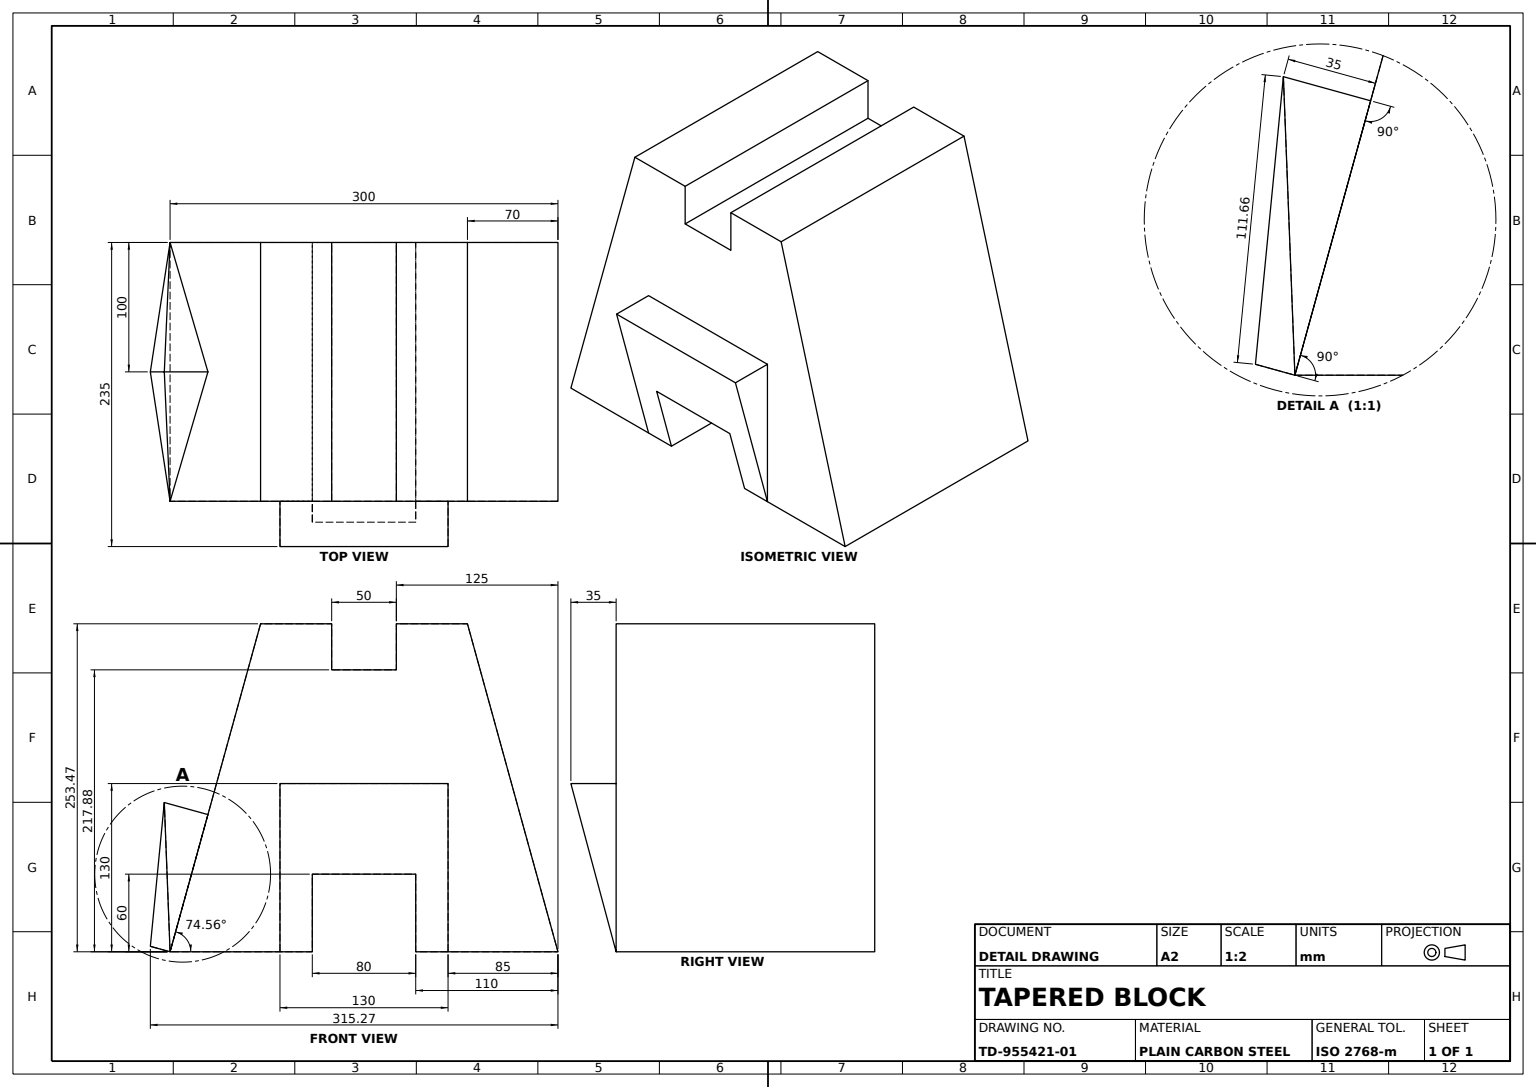
SolidWorks part; units mm, degrees
material "Plain Carbon Steel"
ref_plane "Front Plane" through (0, 0, 0) normal (0, 0, 1) x (1, 0, 0)
ref_plane "Top Plane" through (0, 0, 0) normal (0, 1, 0) x (1, 0, 0)
ref_plane "Right Plane" through (0, 0, 0) normal (1, 0, 0) x (0, 0, -1)
sketch "Pedestal Profile Sketch" plane through (0, 0, 0) normal (0, 0, 1) x (1, 0, 0)
  line L0 (150, 0) -> (150, 287.3946) construction
  line L1 (40, 0) -> (40, 60)
  line L2 (40, 60) -> (-40, 60)
  line L3 (-40, 60) -> (-40, 0)
  line L4 (-40, 0) -> (-150, 0)
  line L5 (-150, 0) -> (-80, 253.468)
  line L6 (-80, 253.468) -> (-25, 253.468)
  line L7 (-25, 253.468) -> (-25, 217.8766)
  line L8 (-25, 217.8766) -> (25, 217.8766)
  line L9 (25, 217.8766) -> (25, 253.468)
  line L10 (25, 253.468) -> (80, 253.468)
  line L11 (80, 253.468) -> (150, 0)
  line L12 (150, 0) -> (40, 0)
  line L13 (-150, 0) -> (-150, 253.468) construction
  dimension "D1" = 300
  dimension "D2" = 70
  dimension "D3" = 55
  dimension "D4" = 50
  dimension "D5" = 55
  dimension "D6" = 70
  dimension "D7" = 40
  dimension "D8" = 150
  dimension "D9" = 40
  dimension "D10" = 150
  dimension "D11" = 253.468
  dimension "D12" = 262.9563
  dimension "D13" = 157.8766
  dimension "D14" = 217.8766
extrude "Pedestal Body" add sketch "Pedestal Profile Sketch" along normal mid plane 200
sketch "Front Boss Sketch" plane through (0, 0, 100) normal (0, 0, 1) x (1, 0, 0)
  line L0 (40, 0) -> (65, 0)
  line L1 (40, 0) -> (150, 0) construction
  line L2 (65, 0) -> (65, 130)
  line L3 (65, 130) -> (-65, 130)
  line L4 (-65, 130) -> (-65, 0)
  line L5 (-150, 0) -> (-40, 0) construction
  line L6 (-65, 0) -> (-40, 0)
  line L7 (-40, 0) -> (-40, 60)
  line L8 (-40, 60) -> (40, 60)
  line L9 (40, 60) -> (40, 0)
  line L10 (-25, 217.8766) -> (-25, 253.468) construction
  dimension "D1" = 90
extrude "Front Boss" add sketch "Front Boss Sketch" along normal blind 35
sketch "Front Boss Cut Sketch" plane through (-65, 0, 0) normal (-1, 0, 0) x (0, 0, 1)
  line L0 (100, 0) -> (135, 130)
  line L1 (100, 0) -> (135, 0)
  line L2 (135, 0) -> (135, 130)
extrude "Front Boss Cut" cut sketch "Front Boss Cut Sketch" against normal through all
sketch "Top Boss Sketch" plane through (-139.3703, 38.4898, 0) normal (-0.9639, 0.2662, 0) x (0, 0, 1)
  line L0 (-100, -39.9306) -> (0, 70.0694)
  line L1 (0, 70.0694) -> (100, -39.9306)
  line L2 (0, -39.9306) -> (0, 70.0694) construction
  line L3 (100, -39.9306) -> (-100, -39.9306) construction
  line L8 (-100, 223.0257) -> (-100, -39.9306)
  line L9 (-100, -39.9306) -> (100, -39.9306)
  line L10 (100, -39.9306) -> (100, 223.0257)
  line L11 (100, 223.0257) -> (-100, 223.0257)
  line L13 (-100, -39.9306) -> (100, -39.9306)
  dimension "D1" = 110
  dimension "D2" = 0
extrude "Top Boss" add sketch "Top Boss Sketch" along normal blind 35
sketch "Top Boss Cut A Sketch" plane through (8.4402, 30.5616, 34.8762) normal (0.1791, 0.6484, 0.7399) x (0.9838, -0.118, -0.1347)
  line L0 (-161.0432, -65.9053) -> (-165.571, 86.7528)
  line L1 (-165.571, 86.7528) -> (-195.3345, -58.8979)
  line L2 (-195.3345, -58.8979) -> (-161.0432, -65.9053)
extrude "Top Boss Cut A" cut sketch "Top Boss Cut A Sketch" against normal through all
sketch "Top Boss Cut B Sketch" plane through (8.4402, 30.5616, -34.8762) normal (0.1791, 0.6484, -0.7399) x (-0.9838, 0.118, -0.1347)
  line L0 (161.0432, -65.9053) -> (165.571, 86.7528)
  line L1 (165.571, 86.7528) -> (192.076, -59.5638)
  line L2 (192.076, -59.5638) -> (161.0432, -65.9053)
extrude "Top Boss Cut B" cut sketch "Top Boss Cut B Sketch" against normal through all
